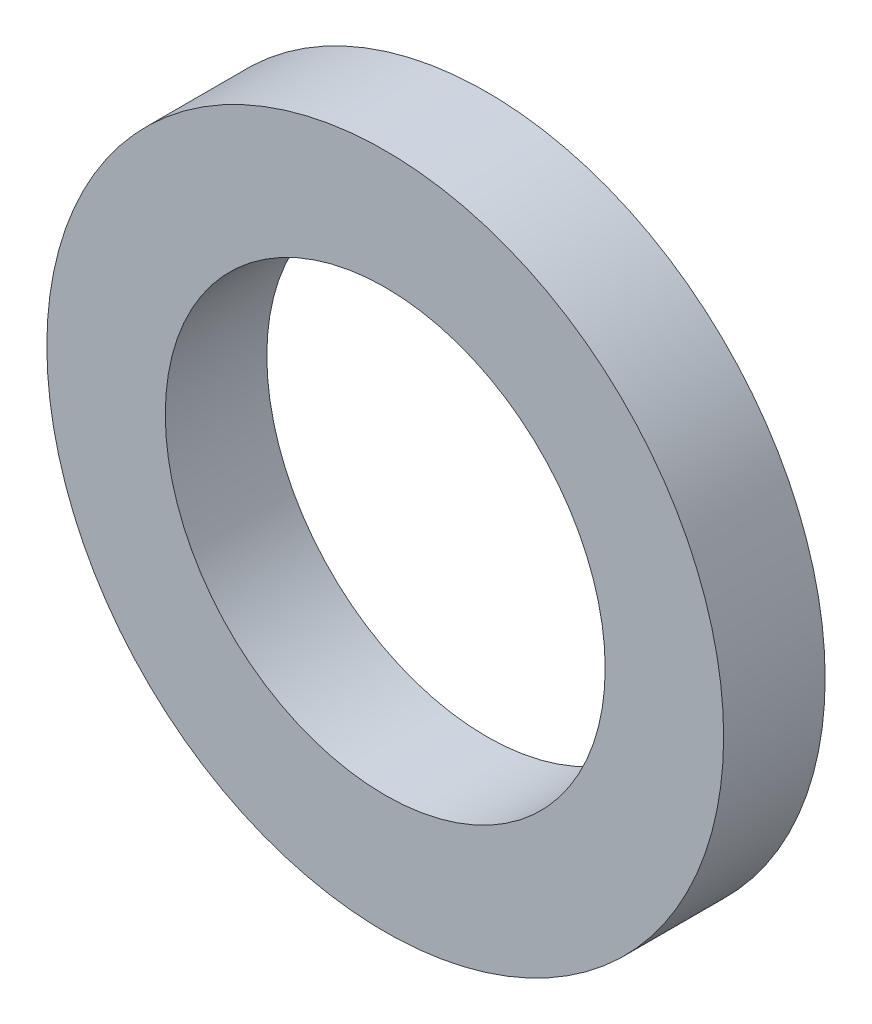
SolidWorks part; units mm, degrees
material "Plain Carbon Steel"
ref_plane "Front Plane" through (0, 0, 0) normal (0, 0, 1) x (1, 0, 0)
ref_plane "Top Plane" through (0, 0, 0) normal (0, 1, 0) x (1, 0, 0)
ref_plane "Right Plane" through (0, 0, 0) normal (1, 0, 0) x (0, 0, -1)
sketch "Washer Profile Ø20xØ13" plane through (0, 0, 0) normal (0, 0, 1) x (1, 0, 0)
  circle A0 centre (0, 0) radius 10
  circle A1 centre (0, 0) radius 6.5
  dimension "D1" = 20
  dimension "D2" = 13
extrude "Washer Body 3mm" add sketch "Washer Profile Ø20xØ13" along normal blind 3
